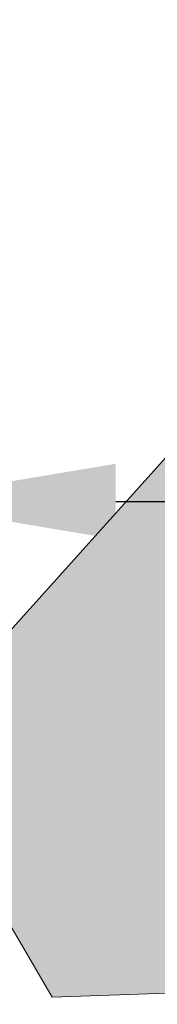
# Model space of a CAD drawing. Units: inches. Extents: x 2091 to 2899, y 967 to 2217.
# Tile 250 of 256: x 2214.58 to 2217.01, y 1131.25 to 1148.63. Entities that reach past the tile are written whole.
import ezdxf

# ---------------------------------------------------------------- set-up
doc = ezdxf.new("R2010")
doc.units = ezdxf.units.IN
doc.layers.add('A-ANNO-DIMS', color=2, linetype='Continuous', lineweight=18)
doc.layers.add('L-PLNT-TREE', color=94, linetype='Continuous', lineweight=13)
doc.layers.add('A-WALL-PATT', color=141, linetype='Continuous', lineweight=13, true_color=0xadddf7)
doc.layers.add('L-PLNT-PATT', color=114, linetype='Continuous', lineweight=13, true_color=0x139b48)
doc.styles.get("Standard").update_dxf_attribs({"font": 'arial.ttf'})
doc.dimstyles.new('ISO-25', dxfattribs={"dimtxt": 4, "dimasz": 4, "dimexe": 1.25, "dimexo": 0.625, "dimtad": 1, "dimdec": 0, "dimlunit": 3, "dimtxsty": 'Standard', "dimcen": 2.5, "dimadec": 0, "dimazin": 0, "dimtfac": 1, "dimtdec": 0, "dimtmove": 0, "dimatfit": 3, "dimfxl": 1, "dimarcsym": 0})

# ---------------------------------------------------------------- blocks, each defined once
blk = doc.blocks.new('*U25')
blk.add_lwpolyline([(-1139.42368, 1783.79628), (-1216.11644, 1685.47796), (-1117.5111, 1601.2033), (-1051.7759, 1643.3419), (-1126.09884, 1521.20092), (-1072.10606, 1527.49758), (-1079.90386, 1416.93646), (-1259.93906, 1179.83508), (-1479.05978, 1165.78888), (-1577.66258, 1109.60662), (-1742.00312, 927.01364), (-1676.26538, 814.64658), (-1270.89408, 828.69278), (-1194.20386, 772.51052), (-1007.95074, 856.78518), (-876.4778, 575.87134), (-821.70016, 575.87134), (-569.71184, 884.87504)])
blk = doc.blocks.new('*D37')
at = {"layer": 'A-ANNO-DIMS', "color": 0, "lineweight": -2, "transparency": 16777216}
for p, q in [((2203.116, 1151.622), (2203.116, 1138.874)), ((2212.276, 1151.622), (2212.276, 1138.874)), ((2199.116, 1140.124), (2195.116, 1140.124)), ((2203.116, 1140.124), (2212.276, 1140.124)), ((2216.276, 1140.124), (2245.908, 1140.124))]:
    blk.add_line(p, q, dxfattribs=at)
at = {"layer": 'A-ANNO-DIMS', "color": 0, "transparency": 16777216}
for points in [[(2199.116, 1140.79), (2199.116, 1139.457), (2203.116, 1140.124)], [(2216.276, 1140.79), (2216.276, 1139.457), (2212.276, 1140.124)]]:
    blk.add_solid(points, dxfattribs=at)
at = {"layer": 'Defpoints', "color": 0, "transparency": 16777216}
for p in [(2203.116, 1152.247), (2212.276, 1152.247), (2212.276, 1140.124)]:
    blk.add_point(p, dxfattribs=at)
at = {"layer": 'A-ANNO-DIMS', "color": 0, "transparency": 16777216, "insert": (2233.092, 1142.791), "char_height": 4, "attachment_point": 5}
blk.add_mtext('0\'-9" TYP.', dxfattribs=at)
blk = doc.blocks.new('*D71')
at = {"layer": 'A-ANNO-DIMS', "color": 0, "lineweight": -2, "transparency": 16777216}
for p, q in [((2212.144, 1351.294), (2212.144, 969.464)), ((2452.144, 1351.294), (2452.144, 969.464)), ((2216.144, 970.714), (2448.144, 970.714))]:
    blk.add_line(p, q, dxfattribs=at)
at = {"layer": 'A-ANNO-DIMS', "color": 0, "transparency": 16777216}
for points in [[(2216.144, 971.381), (2216.144, 970.048), (2212.144, 970.714)], [(2448.144, 971.381), (2448.144, 970.048), (2452.144, 970.714)]]:
    blk.add_solid(points, dxfattribs=at)
at = {"layer": 'Defpoints', "color": 0, "transparency": 16777216}
for p in [(2212.144, 1351.919), (2452.144, 1351.919), (2452.144, 970.714)]:
    blk.add_point(p, dxfattribs=at)
at = {"layer": 'A-ANNO-DIMS', "color": 0, "transparency": 16777216, "insert": (2332.144, 973.382), "char_height": 4, "attachment_point": 5}
blk.add_mtext('20\'-0"', dxfattribs=at)
blk = doc.blocks.new('*D75')
at = {"layer": 'A-ANNO-DIMS', "color": 0, "lineweight": -2, "transparency": 16777216}
for p, q in [((2212.144, 1274.794), (2212.144, 969.464)), ((2308.144, 1274.794), (2308.144, 969.464)), ((2216.144, 970.714), (2304.144, 970.714))]:
    blk.add_line(p, q, dxfattribs=at)
at = {"layer": 'A-ANNO-DIMS', "color": 0, "transparency": 16777216}
for points in [[(2216.144, 971.381), (2216.144, 970.048), (2212.144, 970.714)], [(2304.144, 971.381), (2304.144, 970.048), (2308.144, 970.714)]]:
    blk.add_solid(points, dxfattribs=at)
at = {"layer": 'Defpoints', "color": 0, "transparency": 16777216}
for p in [(2212.144, 1275.419), (2308.144, 1275.419), (2308.144, 970.714)]:
    blk.add_point(p, dxfattribs=at)
at = {"layer": 'A-ANNO-DIMS', "color": 0, "transparency": 16777216, "insert": (2260.144, 973.382), "char_height": 4, "attachment_point": 5}
blk.add_mtext('8\'-0"', dxfattribs=at)

msp = doc.modelspace()

# ---------------------------------------------------------------- hatches: boundary and pattern name
at = {"layer": 'A-WALL-PATT'}
h = msp.add_hatch(color=256, dxfattribs=at)
h.dxf.hatch_style = 1
h.paths.add_polyline_path([(2803.144, 2050.919), (2203.144, 2050.919), (2203.144, 1090.919), (2803.144, 1090.919)])
h.paths.add_polyline_path([(2635.799, 1147.54), (2674.524, 1147.54, 0.376086), (2678.53, 1152.88), (2678.53, 1159.556, 0.333335), (2674.524, 1163.562), (2674.524, 1163.562), (2674.524, 1192.934), (2635.806, 1192.934), (2597.088, 1192.934), (2597.088, 1163.562, 0.333335), (2593.082, 1159.556), (2593.082, 1152.88, 0.376086), (2597.088, 1147.54)], flags=0)
h.paths.add_polyline_path([(2436.01, 1278.241, 0.000483), (2435.953, 1278.215, -0.001328), (2435.936, 1278.112, -0.001711), (2436.116, 1278.041, 0.002185)], flags=0)
h.paths.add_polyline_path([(2794.144, 1143.419), (2794.144, 1347.419), (2543.37, 1347.419), (2543.37, 1351.919), (2794.144, 1351.919), (2794.144, 1392.714), (2793.947, 1392.714), (2793.947, 1473.537), (2794.144, 1473.537), (2794.144, 1531.919), (2650.144, 1531.919), (2650.144, 1536.419), (2794.144, 1536.419), (2794.144, 1692.419), (2609.376, 1692.419), (2609.376, 1644.419), (2604.876, 1644.419), (2604.876, 1744.919), (2609.376, 1744.919), (2609.376, 1696.919), (2794.144, 1696.919), (2794.144, 1780.919), (2609.644, 1780.919), (2493.876, 1780.919), (2493.876, 1785.419), (2609.644, 1785.419), (2794.144, 1785.419), (2794.144, 1847.939), (2793.951, 1847.939), (2793.951, 1928.762), (2794.144, 1928.762), (2794.144, 1941.419), (2614.144, 1941.419), (2614.144, 1821.419), (2609.644, 1821.419), (2609.644, 1941.419), (2392.144, 1941.419), (2392.144, 1819.919), (2387.644, 1819.919), (2387.644, 1941.419), (2212.144, 1941.419), (2212.144, 1783.919), (2392.144, 1783.919), (2392.144, 1780.919), (2212.144, 1780.919), (2212.144, 1629.419), (2387.644, 1629.419), (2387.644, 1744.919), (2392.144, 1744.919), (2392.144, 1627.919), (2317.144, 1627.919), (2317.144, 1551.419), (2317.144, 1536.419), (2459.384, 1536.419), (2459.384, 1602.396), (2463.884, 1602.396), (2463.884, 1531.919), (2456.644, 1531.919), (2456.644, 1529.919), (2452.144, 1529.919), (2452.144, 1531.919), (2312.644, 1531.919), (2312.644, 1551.419), (2306.144, 1551.419), (2306.144, 1555.919), (2308.144, 1555.919), (2308.144, 1551.419), (2312.644, 1551.419), (2312.644, 1627.919), (2212.144, 1627.919), (2212.144, 1555.919), (2270.144, 1555.919), (2270.144, 1551.419), (2212.144, 1551.419), (2212.144, 1351.919), (2272.144, 1351.919), (2272.144, 1347.419), (2212.144, 1347.419), (2212.144, 1275.419), (2308.144, 1275.419), (2308.144, 1351.919), (2452.144, 1351.919), (2452.144, 1493.919), (2456.644, 1493.919), (2456.644, 1347.419), (2312.644, 1347.419), (2312.644, 1270.919), (2212.144, 1270.919), (2212.144, 1099.919), (2281.238, 1099.919), (2282.871, 1110.914), (2282.008, 1116.997), (2278.558, 1121.42), (2268.206, 1128.056), (2272.088, 1128.056), (2273.813, 1131.927), (2279.42, 1134.692), (2285.028, 1135.245), (2287.616, 1137.457), (2288.047, 1138.01), (2289.341, 1140.775), (2291.067, 1139.669), (2292.361, 1135.245), (2295.38, 1136.904), (2296.243, 1135.798), (2297.105, 1133.033), (2300.125, 1138.01), (2303.144, 1138.01), (2304.438, 1135.798), (2303.144, 1133.586), (2306.595, 1134.692), (2307.889, 1133.033), (2310.908, 1135.245), (2313.927, 1134.139), (2315.627, 1132.427), (2308.32, 1117.55), (2290.204, 1109.808), (2288.91, 1103.172), (2289.272, 1099.919), (2434.918, 1099.919), (2431.593, 1124.788), (2429.93, 1169.553), (2430.927, 1240.52), (2435.659, 1238.186), (2437.135, 1196.554), (2438.798, 1143.973), (2442.678, 1111.998), (2446.558, 1099.919), (2794.144, 1099.919), (2794.144, 1138.919), (2548.032, 1138.919), (2548.032, 1143.419), (2548.032, 1148.819), (2546.668, 1148.032), (2528.686, 1179.179, 0.256256), (2512.032, 1148.819), (2512.032, 1143.419), (2512.032, 1138.919), (2507.532, 1138.919), (2507.532, 1143.419), (2507.532, 1148.819, 0.256256), (2490.879, 1179.179), (2472.896, 1148.032), (2471.532, 1148.819), (2471.532, 1143.419), (2467.032, 1143.419), (2467.032, 1269.946, 0.039061), (2460.91, 1273.58), (2467.032, 1273.58), (2467.032, 1286.325, 0.014511), (2465.216, 1286.762), (2467.032, 1287.053), (2467.032, 1323.419), (2471.532, 1323.419), (2471.532, 1148.819), (2489.532, 1179.996), (2490.896, 1179.208), (2490.879, 1179.179, -0.256256), (2507.532, 1148.819), (2507.532, 1143.419), (2512.032, 1143.419), (2512.032, 1148.819, -0.256256), (2528.686, 1179.179), (2528.668, 1179.208), (2530.032, 1179.996), (2548.032, 1148.819), (2548.032, 1143.419)], flags=16)
h.paths.add_polyline_path([(2607.769, 1200.945), (2607.769, 1265.031), (2597.088, 1281.052), (2619.785, 1281.052), (2627.795, 1337.127), (2635.799, 1337.127), (2643.817, 1337.127), (2651.827, 1281.052), (2674.524, 1281.052), (2663.843, 1265.031), (2663.843, 1200.945), (2635.806, 1200.945)], flags=0)
edge = h.paths.add_edge_path(flags=0)
edge.add_ellipse((13303.896, 1272.999), major_axis=(-10595.313, 0), ratio=0.84230387, start_angle=0.6282372, end_angle=0.6465541, ccw=False)
edge.add_ellipse((2711.7, 1156.853), major_axis=(2.22, 0), ratio=0.842304, start_angle=111.5352, end_angle=180.6282, ccw=False)
edge.add_ellipse((13303.156, 1272.999), major_axis=(-10593.026, 0), ratio=0.84230387, start_angle=0.5282715, end_angle=0.6465541, ccw=False)
edge.add_line((2710.765, 1175.333), (2710.13, 1175.333))
edge.add_ellipse((2710.13, 1176.58), major_axis=(1.48, 0), ratio=0.842304, start_angle=180, end_angle=270, ccw=False)
edge.add_line((2708.65, 1176.58), (2708.65, 1200.783))
edge.add_ellipse((2710.13, 1200.783), major_axis=(1.48, 0), ratio=0.842304, start_angle=90, end_angle=180, ccw=False)
edge.add_line((2710.13, 1202.029), (2710.465, 1202.029))
edge.add_ellipse((13303.156, 1272.999), major_axis=(-10593.026, 0), ratio=0.84230387, start_angle=-0.0902291, end_angle=0.3838668, ccw=False)
edge.add_ellipse((2710.13, 1290.927), major_axis=(-1.48, 0), ratio=0.842304, start_angle=0, end_angle=90, ccw=False)
edge.add_line((2708.65, 1290.927), (2708.65, 1315.13))
edge.add_ellipse((2710.13, 1315.13), major_axis=(-1.48, 0), ratio=0.842304, start_angle=-90, end_angle=0, ccw=False)
edge.add_line((2710.13, 1316.377), (2710.706, 1316.377))
edge.add_ellipse((3238.402, 1296.29), major_axis=(528.234, 0), ratio=0.8423039, start_angle=176.34957, end_angle=177.82005, ccw=False)
edge.add_ellipse((2775.063, 1071.451), major_axis=(313.308, 0), ratio=0.8423039, start_angle=102.12597, end_angle=103.78053, ccw=False)
edge.add_ellipse((2775.063, 1078.306), major_axis=(-305.303, 0), ratio=0.8423039, start_angle=-79.79046, end_angle=-77.55537, ccw=False)
edge.add_ellipse((2695.142, 1541.975), major_axis=(-250.96, 0), ratio=0.8423039, start_angle=99.25657, end_angle=102.55493)
edge.add_line((2741.41, 1334.214), (2747.133, 1337.378))
edge.add_ellipse((2747.539, 1336.857), major_axis=(-0.74, 0), ratio=0.842304, start_angle=270, end_angle=307.9331, ccw=False)
edge.add_ellipse((2747.539, 1336.857), major_axis=(-0.74, 0), ratio=0.842304, start_angle=232.0669, end_angle=270, ccw=False)
edge.add_line((2747.945, 1337.378), (2753.667, 1334.214))
edge.add_ellipse((2799.935, 1541.975), major_axis=(250.96, 0), ratio=0.8423039, start_angle=257.44507, end_angle=260.74343)
edge.add_ellipse((2720.014, 1078.306), major_axis=(305.303, 0), ratio=0.8423039, start_angle=77.55537, end_angle=79.79046, ccw=False)
edge.add_ellipse((2720.014, 1071.451), major_axis=(-313.308, 0), ratio=0.8423039, start_angle=256.21947, end_angle=257.87403, ccw=False)
edge.add_ellipse((2256.676, 1296.29), major_axis=(-528.234, 0), ratio=0.8423039, start_angle=182.17995, end_angle=183.65043, ccw=False)
edge.add_line((2784.371, 1316.377), (2784.947, 1316.377))
edge.add_ellipse((2784.947, 1315.13), major_axis=(1.48, 0), ratio=0.842304, start_angle=0, end_angle=90, ccw=False)
edge.add_line((2786.427, 1315.13), (2786.427, 1290.927))
edge.add_ellipse((2784.947, 1290.927), major_axis=(1.48, 0), ratio=0.842304, start_angle=270, end_angle=360, ccw=False)
edge.add_ellipse((-7808.079, 1272.999), major_axis=(10593.026, 0), ratio=0.84230387, start_angle=-0.3838668, end_angle=0.0902291, ccw=False)
edge.add_line((2784.612, 1202.029), (2784.947, 1202.029))
edge.add_ellipse((2784.947, 1200.783), major_axis=(1.48, 0), ratio=0.842304, start_angle=0, end_angle=90, ccw=False)
edge.add_line((2786.427, 1200.783), (2786.427, 1176.58))
edge.add_ellipse((2784.947, 1176.58), major_axis=(-1.48, 0), ratio=0.842304, start_angle=90, end_angle=180, ccw=False)
edge.add_line((2784.947, 1175.333), (2784.313, 1175.333))
edge.add_ellipse((-7808.079, 1272.999), major_axis=(10593.026, 0), ratio=0.84230387, start_angle=-0.6186432, end_angle=-0.5282715, ccw=False)
edge.add_ellipse((2783.377, 1156.853), major_axis=(-2.22, 0), ratio=0.842304, start_angle=179.3718, end_angle=248.4648, ccw=False)
edge.add_ellipse((-7808.819, 1272.999), major_axis=(-10595.313, 0), ratio=0.842303866, start_angle=179.3534459, end_angle=179.3717628, ccw=False)
edge.add_ellipse((2780.297, 1153.501), major_axis=(-5.246, 0), ratio=0.842304, start_angle=90, end_angle=179.3534, ccw=False)
edge.add_line((2780.297, 1149.082), (2714.78, 1149.082))
edge.add_ellipse((2714.78, 1153.501), major_axis=(5.246, 0), ratio=0.842304, start_angle=180.6466, end_angle=270, ccw=False)
edge = h.paths.add_edge_path(flags=0)
edge.add_line((2718.187, 1151.008), (2718.187, 1170.472))
edge.add_ellipse((2721.147, 1170.472), major_axis=(-2.96, 0), ratio=0.842304, start_angle=-90, end_angle=0, ccw=False)
edge.add_line((2721.147, 1172.965), (2773.93, 1172.965))
edge.add_ellipse((2773.93, 1170.472), major_axis=(-2.96, 0), ratio=0.842304, start_angle=180, end_angle=270, ccw=False)
edge.add_line((2776.89, 1170.472), (2776.89, 1151.008))
edge.add_line((2776.89, 1151.008), (2718.187, 1151.008))
edge = h.paths.add_edge_path(flags=0)
edge.add_line((2718.187, 1180.234), (2718.187, 1199.058))
edge.add_ellipse((2747.539, 1320.399), major_axis=(147.018, 0), ratio=0.8423039, start_angle=256.40187, end_angle=283.59813)
edge.add_line((2776.89, 1199.058), (2776.89, 1180.234))
edge.add_ellipse((2747.539, 1301.575), major_axis=(147.018, 0), ratio=0.8423039, start_angle=256.40187, end_angle=283.59813, ccw=False)
edge = h.paths.add_edge_path(flags=0)
edge.add_ellipse((13303.156, 1272.999), major_axis=(-10591.546, 0), ratio=0.84230387, start_angle=0.0555943, end_angle=0.3777642, ccw=False)
edge.add_line((2711.617, 1262.722), (2715.667, 1249.495))
edge.add_ellipse((6413.892, 1241.692), major_axis=(-3698.236, 0), ratio=0.84230387, start_angle=-0.120897, end_angle=0.364076)
edge.add_line((2715.761, 1218.192), (2711.934, 1203.167))
edge = h.paths.add_edge_path(flags=0)
edge.add_line((2718.187, 1251.075), (2716.002, 1267.45))
edge.add_ellipse((2742.151, 1202.19), major_axis=(81.773, 0), ratio=0.842304, start_angle=94.27742, end_angle=111.83495, ccw=False)
edge.add_line((2737.01, 1270.931), (2758.067, 1270.931))
edge.add_ellipse((2752.926, 1202.19), major_axis=(81.773, 0), ratio=0.842304, start_angle=68.16505, end_angle=85.72258, ccw=False)
edge.add_line((2779.075, 1267.45), (2776.89, 1251.075))
edge.add_ellipse((2750.338, 1187.885), major_axis=(79.58, 0), ratio=0.842304, start_angle=67.20809, end_angle=85.12993)
edge.add_line((2756.035, 1254.744), (2739.043, 1254.744))
edge.add_ellipse((2744.739, 1187.885), major_axis=(79.58, 0), ratio=0.842304, start_angle=94.87007, end_angle=112.79191)
edge = h.paths.add_edge_path(flags=0)
edge.add_line((2783.143, 1203.167), (2779.316, 1218.192))
edge.add_ellipse((-918.815, 1241.692), major_axis=(3698.236, 0), ratio=0.84230387, start_angle=-0.364076, end_angle=0.120897)
edge.add_line((2779.41, 1249.495), (2783.46, 1262.722))
edge.add_ellipse((-7808.079, 1272.999), major_axis=(-10591.546, 0), ratio=0.84230387, start_angle=179.6222358, end_angle=179.9444057, ccw=False)
edge = h.paths.add_edge_path(flags=0)
edge.add_ellipse((2734.201, 1286.69), major_axis=(-0.357, 6.34), ratio=0.603834, start_angle=89.002, end_angle=253.6574, ccw=False)
edge.add_line((2730.369, 1286.542), (2730.369, 1301.352))
edge.add_line((2730.369, 1301.352), (2735.913, 1305.215))
edge.add_ellipse((2736.385, 1304.735), major_axis=(0.74, 0), ratio=0.842304, start_angle=90, end_angle=134.4802, ccw=False)
edge.add_line((2736.385, 1305.358), (2738.033, 1305.358))
edge.add_line((2738.033, 1305.358), (2738.033, 1307.708))
edge.add_ellipse((2794.202, 1307.708), major_axis=(56.169, 0), ratio=0.842304, start_angle=150.5614, end_angle=180, ccw=False)
edge.add_ellipse((2700.876, 1307.708), major_axis=(-56.169, 0), ratio=0.842304, start_angle=180, end_angle=209.4386, ccw=False)
edge.add_line((2757.044, 1307.708), (2757.044, 1305.358))
edge.add_line((2757.044, 1305.358), (2758.692, 1305.358))
edge.add_ellipse((2758.692, 1304.735), major_axis=(-0.74, 0), ratio=0.842304, start_angle=225.5198, end_angle=270, ccw=False)
edge.add_line((2759.164, 1305.215), (2764.708, 1301.352))
edge.add_line((2764.708, 1301.352), (2764.708, 1286.542))
edge.add_ellipse((2760.876, 1286.69), major_axis=(0.357, 6.34), ratio=0.603834, start_angle=106.3426, end_angle=270.998, ccw=False)
edge.add_line((2757.044, 1285.797), (2757.044, 1307.708))
edge.add_ellipse((2700.876, 1307.708), major_axis=(-56.169, 0), ratio=0.842304, start_angle=180, end_angle=209.4386)
edge.add_ellipse((2794.202, 1307.708), major_axis=(56.169, 0), ratio=0.842304, start_angle=150.5614, end_angle=180)
edge.add_line((2738.033, 1307.708), (2738.033, 1285.797))
h.paths.add_polyline_path([(2417.812, 1104.45), (2413.492, 1102.53), (2410.612, 1103.97), (2409.172, 1106.37), (2407.252, 1107.33), (2406.292, 1109.73), (2405.332, 1114.05), (2405.332, 1117.89), (2406.292, 1120.13), (2407.252, 1119.81), (2408.848, 1118.328), (2410.174, 1119.424), (2410.211, 1120.406), (2411.041, 1121.419), (2410.699, 1119.859), (2410.174, 1119.424), (2410.088, 1117.176), (2411.133, 1116.206), (2413.972, 1119.33), (2416.852, 1120.77), (2416.87, 1120.799), (2417.035, 1119.405), (2417.896, 1118.143), (2418.292, 1118.37), (2419.544, 1120.039), (2419.361, 1118.387), (2419.032, 1119.356), (2418.399, 1118.512), (2419.252, 1114.53), (2418.794, 1107.199)], flags=0)
h.paths.add_polyline_path([(2508.87, 1347.419), (2508.37, 1347.419), (2508.37, 1351.919), (2508.87, 1351.919)], flags=0)
h.paths.add_polyline_path([(2473.37, 1347.419), (2472.37, 1347.419), (2467.87, 1347.419), (2467.87, 1455.419), (2472.37, 1455.419), (2472.37, 1352.419), (2473.37, 1352.419)], flags=0)
h.paths.add_polyline_path([(2352.106, 1217.446), (2349.226, 1218.886), (2347.786, 1221.286), (2345.866, 1222.246), (2344.906, 1224.646), (2343.946, 1228.966), (2343.946, 1232.806), (2344.906, 1235.046), (2345.866, 1234.726), (2347.462, 1233.244), (2348.788, 1234.341), (2348.825, 1235.322), (2349.655, 1236.336), (2349.313, 1234.775), (2348.788, 1234.341), (2348.702, 1232.093), (2349.747, 1231.123), (2352.586, 1234.246), (2355.466, 1235.686), (2355.484, 1235.715), (2355.649, 1234.322), (2356.51, 1233.06), (2356.906, 1233.286), (2358.158, 1234.956), (2357.975, 1233.304), (2357.646, 1234.273), (2357.013, 1233.428), (2357.866, 1229.446), (2357.408, 1222.115), (2356.426, 1219.366)], flags=0)
h.paths.add_polyline_path([(2348.297, 1112.224), (2347.014, 1112.31), (2345.53, 1114.127), (2345.732, 1115.858), (2346.812, 1116.982), (2346.812, 1114.646), (2345.867, 1114.214), (2346.88, 1114.3)], flags=0)
h.paths.add_polyline_path([(2347.014, 1110.926), (2346.272, 1110.493), (2346.61, 1111.186)], flags=0)
h.paths.add_polyline_path([(2345.867, 1118.194), (2345.53, 1117.329), (2343.708, 1118.021), (2344.383, 1118.626)], flags=0)
h.paths.add_polyline_path([(2346.677, 1109.282), (2346.07, 1108.071), (2345.867, 1110.061)], flags=0)
h.paths.add_polyline_path([(2345.057, 1119.751), (2343.64, 1119.751), (2343.978, 1121.135)], flags=0)
h.paths.add_polyline_path([(2345.26, 1116.55), (2345.125, 1115.858), (2344.922, 1115.685), (2344.72, 1116.377)], flags=0)
h.paths.add_polyline_path([(2345.665, 1112.31), (2345.462, 1111.532), (2344.045, 1111.964), (2344.652, 1112.57)], flags=0)
h.paths.add_polyline_path([(2345.192, 1113.349), (2344.45, 1113.868), (2344.72, 1114.387)], flags=0)
h.paths.add_polyline_path([(2344.652, 1116.809), (2344.18, 1115.685), (2344.652, 1115.339), (2343.91, 1114.906), (2343.033, 1115.944), (2343.64, 1116.463)], flags=0)
h.paths.add_polyline_path([(2345.867, 1106.686), (2344.99, 1105.562), (2344.517, 1106.6)], flags=0)
h.paths.add_polyline_path([(2344.855, 1110.061), (2344.517, 1109.282), (2344.113, 1109.715)], flags=0)
h.paths.add_polyline_path([(2344.045, 1113.522), (2343.438, 1113.089), (2342.763, 1113.954)], flags=0)
h.paths.add_polyline_path([(2344.315, 1111.012), (2342.965, 1110.32), (2342.965, 1111.099)], flags=0)
h.paths.add_polyline_path([(2345.125, 1104.697), (2344.585, 1103.745), (2344.45, 1104.264)], flags=0)
h.paths.add_polyline_path([(2342.83, 1121.222), (2341.75, 1120.53), (2340.536, 1121.049), (2340.131, 1121.828), (2340.671, 1122.952), (2341.143, 1121.828), (2341.615, 1122.001)], flags=0)
h.paths.add_polyline_path([(2342.965, 1119.751), (2343.033, 1118.453), (2342.088, 1118.021), (2342.02, 1119.491)], flags=0)
h.paths.add_polyline_path([(2342.695, 1116.896), (2341.953, 1116.636), (2342.02, 1117.329)], flags=0)
h.paths.add_polyline_path([(2343.033, 1112.224), (2342.02, 1111.791), (2341.548, 1112.224), (2342.358, 1113.349)], flags=0)
h.paths.add_polyline_path([(2343.775, 1104.437), (2342.628, 1102.88), (2342.695, 1104.61), (2343.438, 1105.129)], flags=0)
h.paths.add_polyline_path([(2342.02, 1115.079), (2340.806, 1115.512), (2340.941, 1116.377)], flags=0)
h.paths.add_polyline_path([(2341.481, 1120.097), (2341.481, 1119.405), (2341.076, 1119.578), (2341.143, 1120.097)], flags=0)
h.paths.add_polyline_path([(2341.818, 1114.473), (2340.941, 1113.089), (2340.806, 1114.56)], flags=0)
h.paths.add_polyline_path([(2341.143, 1118.54), (2340.941, 1116.982), (2339.051, 1117.675), (2339.051, 1118.626)], flags=0)
h.paths.add_polyline_path([(2342.695, 1101.668), (2341.953, 1101.841), (2342.56, 1102.361)], flags=0)
h.paths.add_polyline_path([(2340.333, 1119.665), (2338.444, 1119.578), (2337.904, 1120.357), (2339.658, 1120.616)], flags=0)
h.paths.add_polyline_path([(2340.333, 1115.339), (2340.063, 1113.695), (2339.388, 1115.339)], flags=0)
h.paths.add_polyline_path([(2341.818, 1103.831), (2341.548, 1102.88), (2341.143, 1103.658)], flags=0)
h.paths.add_polyline_path([(2339.051, 1122.866), (2337.296, 1121.828), (2337.094, 1123.125), (2337.769, 1123.818)], flags=0)
h.paths.add_polyline_path([(2339.118, 1121.741), (2338.848, 1121.222), (2338.174, 1121.049), (2338.376, 1121.568)], flags=0)
h.paths.add_polyline_path([(2339.186, 1119.319), (2338.646, 1118.713), (2338.241, 1118.107), (2338.241, 1118.886)], flags=0)
h.paths.add_polyline_path([(2341.143, 1101.928), (2340.603, 1101.236), (2340.063, 1101.841), (2340.603, 1102.361)], flags=0)
h.paths.add_polyline_path([(2337.634, 1117.761), (2336.621, 1118.28), (2337.296, 1118.972)], flags=0)
h.paths.add_polyline_path([(2336.824, 1119.578), (2334.799, 1118.972), (2335.204, 1120.357), (2336.554, 1120.876)], flags=0)
h.paths.add_polyline_path([(2339.118, 1100.457), (2337.364, 1100.543), (2336.756, 1101.236)], flags=0)
h.paths.add_polyline_path([(2336.351, 1122.433), (2336.014, 1121.914), (2334.934, 1122.433), (2334.529, 1123.471), (2335.744, 1122.779)], flags=0)
h.paths.add_polyline_path([(2334.732, 1120.876), (2334.259, 1120.357), (2334.057, 1120.789), (2334.597, 1121.308)], flags=0)
h.paths.add_polyline_path([(2334.462, 1122.174), (2332.572, 1121.308), (2331.357, 1122.174), (2332.1, 1122.866)], flags=0)
h.paths.add_polyline_path([(2334.259, 1118.54), (2333.382, 1118.453), (2333.652, 1119.319)], flags=0)
h.paths.add_polyline_path([(2335.542, 1102.274), (2334.192, 1102.62), (2335.272, 1103.312)], flags=0)
h.paths.add_polyline_path([(2332.707, 1119.665), (2331.695, 1120.443), (2332.505, 1120.789)], flags=0)
h.paths.add_polyline_path([(2334.732, 1101.149), (2333.517, 1101.582), (2333.989, 1101.755)], flags=0)
h.paths.add_polyline_path([(2332.64, 1116.636), (2331.087, 1116.29), (2331.965, 1118.194)], flags=0)
h.paths.add_polyline_path([(2330.75, 1121.568), (2330.277, 1120.27), (2328.523, 1119.319), (2328.995, 1121.049)], flags=0)
h.paths.add_polyline_path([(2330.75, 1118.626), (2330.008, 1117.502), (2329.873, 1118.021)], flags=0)
h.paths.add_polyline_path([(2332.1, 1102.361), (2330.547, 1102.014), (2331.695, 1102.966)], flags=0)
h.paths.add_polyline_path([(2329.535, 1113.608), (2329.063, 1112.31), (2328.59, 1113.349)], flags=0)
h.paths.add_polyline_path([(2328.388, 1117.848), (2327.51, 1116.55), (2327.173, 1117.761)], flags=0)
h.paths.add_polyline_path([(2329.738, 1106.513), (2329.535, 1105.302), (2328.253, 1106.081)], flags=0)
h.paths.add_polyline_path([(2328.658, 1114.387), (2328.05, 1114.127), (2328.32, 1114.906)], flags=0)
h.paths.add_polyline_path([(2328.32, 1112.224), (2327.106, 1112.137), (2326.701, 1112.656)], flags=0)
h.paths.add_polyline_path([(2326.903, 1115.252), (2326.701, 1114.127), (2325.216, 1113.608), (2326.093, 1115.339)], flags=0)
h.paths.add_polyline_path([(2326.633, 1108.33), (2326.093, 1107.379), (2325.891, 1108.503), (2326.498, 1109.109)], flags=0)
h.paths.add_polyline_path([(2615.144, 1531.919), (2609.644, 1531.919), (2609.644, 1620.419), (2614.144, 1620.419), (2614.144, 1536.419), (2615.144, 1536.419)], flags=0)
h.paths.add_polyline_path([(2545.144, 1563.419), (2464.144, 1563.419), (2464.144, 1632.419), (2509.144, 1632.419), (2509.144, 1627.919), (2509.144, 1603.919), (2468.644, 1603.919), (2468.644, 1567.919), (2540.644, 1567.919), (2540.644, 1591.919), (2545.144, 1591.919)], flags=0)
h.paths.add_polyline_path([(2388.969, 1549.986), (2357.434, 1549.986), (2357.434, 1623.361), (2399.363, 1623.361), (2435.689, 1623.361), (2435.593, 1602.559), (2435.593, 1602.396), (2388.969, 1602.396)], flags=0)
h.paths.add_polyline_path([(2388.881, 1555.809), (2374.904, 1555.809), (2374.904, 1600.572), (2374.904, 1615.458), (2406.351, 1615.458), (2406.351, 1618.939), (2412.174, 1615.458), (2406.351, 1611.976), (2406.351, 1615.458), (2388.881, 1615.458)], flags=0)
h.paths.add_polyline_path([(2568.876, 1644.419), (2453.376, 1644.419), (2453.376, 1785.419), (2457.876, 1785.419), (2457.876, 1648.919), (2568.876, 1648.919)], flags=0)
h.paths.add_polyline_path([(2212.144, 1945.919), (2212.144, 2041.919), (2794.144, 2041.919), (2794.144, 1945.919)], flags=16)
h.paths.add_polyline_path([(2271.083, 1964.317), (2776.853, 1964.317), (2776.853, 2037.17), (2271.083, 2037.17)], flags=8)
h.paths.add_polyline_path([(2380.649, 1536.824), (2461.041, 1536.824), (2461.041, 1554.653), (2380.649, 1554.653)], flags=8)
h.paths.add_polyline_path([(2240.756, 1609.725), (2309.186, 1609.725), (2309.186, 1617.698), (2240.756, 1617.698)], flags=8)
h.paths.add_polyline_path([(2212.677, 1313.504), (2282.592, 1313.504), (2282.592, 1322.745), (2212.677, 1322.745)], flags=8)
h.paths.add_polyline_path([(2457.112, 1114.779), (2558.482, 1114.779), (2558.482, 1142.22), (2457.112, 1142.22)], flags=8)
h.paths.add_polyline_path([(2473.442, 1273.01), (2604.641, 1273.01), (2604.641, 1318.347), (2473.442, 1318.347)], flags=8)
h.paths.add_polyline_path([(2638.876, 1626.977), (2684.25, 1627.977), (2684.038, 1637.597), (2638.664, 1636.598)], flags=8)
h.paths.add_polyline_path([(2537.591, 1453.793), (2628.39, 1453.793), (2628.39, 1475.345), (2537.591, 1475.345)], flags=8)
h.paths.add_polyline_path([(2504.138, 1714.632), (2554.647, 1714.632), (2554.647, 1730.238), (2504.138, 1730.238)], flags=8)
h.paths.add_polyline_path([(2487.501, 1575.652), (2535.097, 1575.652), (2535.097, 1598.378), (2487.501, 1598.378)], flags=8)
h.paths.add_polyline_path([(2709.099, 1735.71), (2740.017, 1735.71), (2740.017, 1749.938), (2709.099, 1749.938)], flags=8)
h.paths.add_polyline_path([(2442.438, 1792.172), (2564.729, 1792.172), (2564.729, 1842), (2442.438, 1842)], flags=8)
h.paths.add_polyline_path([(2655.816, 1809.644), (2789.52, 1806.694), (2790.085, 1832.292), (2656.381, 1835.242)], flags=8)
h.paths.add_polyline_path([(2234.843, 1797.72), (2368.593, 1794.769), (2369.161, 1820.504), (2235.411, 1823.455)], flags=8)
h.paths.add_polyline_path([(2245.138, 1644.006), (2398.428, 1640.624), (2398.995, 1666.325), (2245.706, 1669.707)], flags=8)
h.paths.add_polyline_path([(2306.143, 1431.169), (2413.768, 1428.794), (2414.333, 1454.392), (2306.708, 1456.766)], flags=8)
h.paths.add_polyline_path([(2306.835, 1458.233), (2393.38, 1456.323), (2393.933, 1481.354), (2307.387, 1483.264)], flags=8)
at = {"layer": 'L-PLNT-PATT'}
h = msp.add_hatch(color=256, dxfattribs=at)
h.dxf.hatch_style = 1
h.paths.add_polyline_path([(2333.338, 1165.659), (2329.024, 1166.212), (2331.612, 1168.424), (2335.063, 1177.271), (2328.162, 1184.46), (2319.535, 1187.225), (2323.417, 1193.308), (2319.966, 1203.814), (2317.809, 1203.814), (2313.496, 1213.215), (2310.908, 1212.662), (2307.889, 1212.662), (2305.732, 1217.086), (2307.026, 1223.168), (2310.477, 1223.168), (2304.007, 1230.91), (2303.136, 1237.046), (2299.693, 1240.864), (2296.674, 1237.546), (2294.949, 1238.652), (2294.517, 1241.417), (2292.361, 1242.523), (2289.341, 1239.758), (2285.89, 1240.311), (2283.302, 1235.334), (2283.302, 1230.91), (2286.753, 1229.251), (2284.165, 1227.592), (2281.577, 1229.804), (2274.244, 1222.615), (2274.244, 1220.957), (2271.225, 1219.298), (2272.088, 1217.639), (2274.244, 1214.321), (2270.362, 1211.556), (2266.48, 1214.321), (2264.324, 1213.768), (2263.461, 1211.556), (2266.48, 1211.003), (2266.912, 1206.579), (2263.539, 1207.132), (2259.579, 1203.261), (2263.892, 1202.708), (2262.167, 1197.178), (2258.285, 1196.625), (2253.971, 1193.861), (2248.795, 1191.096), (2248.364, 1193.308), (2244.482, 1185.013), (2251.383, 1186.672), (2255.697, 1183.907), (2254.403, 1177.271), (2246.639, 1174.506), (2243.188, 1176.718), (2241.894, 1173.4), (2238.875, 1172.847), (2236.287, 1169.53), (2233.267, 1165.659), (2237.149, 1162.341), (2239.737, 1164), (2236.811, 1159.191), (2238.937, 1159.439), (2238.63, 1155.086), (2231.542, 1145.752), (2222.915, 1145.199), (2219.033, 1142.987), (2212.563, 1135.798), (2215.151, 1131.374), (2231.111, 1131.927), (2234.13, 1129.715), (2241.463, 1133.033), (2246.639, 1121.973), (2248.795, 1121.973), (2258.716, 1134.139), (2261.736, 1135.798), (2263.892, 1133.033), (2263.892, 1129.162), (2267.343, 1128.056), (2272.088, 1128.056), (2273.813, 1131.927), (2279.42, 1134.692), (2285.028, 1135.245), (2287.616, 1137.457), (2288.047, 1138.01), (2289.341, 1140.775), (2291.067, 1139.669), (2292.361, 1135.245), (2295.38, 1136.904), (2296.243, 1135.798), (2297.105, 1133.033), (2300.125, 1138.01), (2303.144, 1138.01), (2304.438, 1135.798), (2303.144, 1133.586), (2306.595, 1134.692), (2307.889, 1133.033), (2310.908, 1135.245), (2313.927, 1134.139), (2319.966, 1128.056), (2322.554, 1126.95), (2324.711, 1124.738), (2342.827, 1126.397), (2346.278, 1123.079), (2348.866, 1124.185), (2341.964, 1133.033), (2341.533, 1136.351), (2343.69, 1139.669), (2339.808, 1150.175), (2337.651, 1150.175)])
h.paths.add_polyline_path([(2339.658, 1120.616), (2337.904, 1120.357), (2338.444, 1119.578), (2340.333, 1119.665)])
h.paths.add_polyline_path([(2341.143, 1118.54), (2339.051, 1118.626), (2339.051, 1117.675), (2340.941, 1116.982)])
h.paths.add_polyline_path([(2336.554, 1120.876), (2335.204, 1120.357), (2334.799, 1118.972), (2336.824, 1119.578)])
h.paths.add_polyline_path([(2337.296, 1118.972), (2336.621, 1118.28), (2337.634, 1117.761)])
h.paths.add_polyline_path([(2338.646, 1118.713), (2339.186, 1119.319), (2338.241, 1118.886), (2338.241, 1118.107)])
h.paths.add_polyline_path([(2339.051, 1122.866), (2337.769, 1123.818), (2337.094, 1123.125), (2337.296, 1121.828)])
h.paths.add_polyline_path([(2341.615, 1122.001), (2341.143, 1121.828), (2340.671, 1122.952), (2340.131, 1121.828), (2340.536, 1121.049), (2341.75, 1120.53), (2342.83, 1121.222)])
h.paths.add_polyline_path([(2342.965, 1119.751), (2342.02, 1119.491), (2342.088, 1118.021), (2343.033, 1118.453)])
h.paths.add_polyline_path([(2345.867, 1118.194), (2344.383, 1118.626), (2343.708, 1118.021), (2345.53, 1117.329)])
h.paths.add_polyline_path([(2344.652, 1116.809), (2343.64, 1116.463), (2343.033, 1115.944), (2343.91, 1114.906), (2344.652, 1115.339), (2344.18, 1115.685)])
h.paths.add_polyline_path([(2346.812, 1116.982), (2345.732, 1115.858), (2345.53, 1114.127), (2347.014, 1112.31), (2348.297, 1112.224), (2346.88, 1114.3), (2345.867, 1114.214), (2346.812, 1114.646)])
h.paths.add_polyline_path([(2345.26, 1116.55), (2344.72, 1116.377), (2344.922, 1115.685), (2345.125, 1115.858)])
h.paths.add_polyline_path([(2342.695, 1116.896), (2342.02, 1117.329), (2341.953, 1116.636)])
h.paths.add_polyline_path([(2341.481, 1120.097), (2341.143, 1120.097), (2341.076, 1119.578), (2341.481, 1119.405)])
h.paths.add_polyline_path([(2343.978, 1121.135), (2343.64, 1119.751), (2345.057, 1119.751)])
h.paths.add_polyline_path([(2339.118, 1121.741), (2338.376, 1121.568), (2338.174, 1121.049), (2338.848, 1121.222)])
h.paths.add_polyline_path([(2336.351, 1122.433), (2335.744, 1122.779), (2334.529, 1123.471), (2334.934, 1122.433), (2336.014, 1121.914)])
h.paths.add_polyline_path([(2334.462, 1122.174), (2332.1, 1122.866), (2331.357, 1122.174), (2332.572, 1121.308)])
h.paths.add_polyline_path([(2334.597, 1121.308), (2334.057, 1120.789), (2334.259, 1120.357), (2334.732, 1120.876)])
h.paths.add_polyline_path([(2332.505, 1120.789), (2331.695, 1120.443), (2332.707, 1119.665)])
h.paths.add_polyline_path([(2333.652, 1119.319), (2333.382, 1118.453), (2334.259, 1118.54)])
h.paths.add_polyline_path([(2331.965, 1118.194), (2331.087, 1116.29), (2332.64, 1116.636)])
h.paths.add_polyline_path([(2330.75, 1121.568), (2328.995, 1121.049), (2328.523, 1119.319), (2330.277, 1120.27)])
h.paths.add_polyline_path([(2330.75, 1118.626), (2329.873, 1118.021), (2330.008, 1117.502)])
h.paths.add_polyline_path([(2328.388, 1117.848), (2327.173, 1117.761), (2327.51, 1116.55)])
h.paths.add_polyline_path([(2326.903, 1115.252), (2326.093, 1115.339), (2325.216, 1113.608), (2326.701, 1114.127)])
h.paths.add_polyline_path([(2328.658, 1114.387), (2328.32, 1114.906), (2328.05, 1114.127)])
h.paths.add_polyline_path([(2326.701, 1112.656), (2327.106, 1112.137), (2328.32, 1112.224)])
h.paths.add_polyline_path([(2329.535, 1113.608), (2328.59, 1113.349), (2329.063, 1112.31)])
h.paths.add_polyline_path([(2340.333, 1115.339), (2339.388, 1115.339), (2340.063, 1113.695)])
h.paths.add_polyline_path([(2340.941, 1116.377), (2340.806, 1115.512), (2342.02, 1115.079)])
h.paths.add_polyline_path([(2341.818, 1114.473), (2340.806, 1114.56), (2340.941, 1113.089)])
h.paths.add_polyline_path([(2343.033, 1112.224), (2342.358, 1113.349), (2341.548, 1112.224), (2342.02, 1111.791)])
h.paths.add_polyline_path([(2342.763, 1113.954), (2343.438, 1113.089), (2344.045, 1113.522)])
h.paths.add_polyline_path([(2344.72, 1114.387), (2344.45, 1113.868), (2345.192, 1113.349)])
h.paths.add_polyline_path([(2345.665, 1112.31), (2344.652, 1112.57), (2344.045, 1111.964), (2345.462, 1111.532)])
h.paths.add_polyline_path([(2344.315, 1111.012), (2342.965, 1111.099), (2342.965, 1110.32)])
h.paths.add_polyline_path([(2344.855, 1110.061), (2344.113, 1109.715), (2344.517, 1109.282)])
h.paths.add_polyline_path([(2346.677, 1109.282), (2345.867, 1110.061), (2346.07, 1108.071)])
h.paths.add_polyline_path([(2347.014, 1110.926), (2346.61, 1111.186), (2346.272, 1110.493)])
h.paths.add_polyline_path([(2345.867, 1106.686), (2344.517, 1106.6), (2344.99, 1105.562)])
h.paths.add_polyline_path([(2345.125, 1104.697), (2344.45, 1104.264), (2344.585, 1103.745)])
h.paths.add_polyline_path([(2343.775, 1104.437), (2343.438, 1105.129), (2342.695, 1104.61), (2342.628, 1102.88)])
h.paths.add_polyline_path([(2341.818, 1103.831), (2341.143, 1103.658), (2341.548, 1102.88)])
h.paths.add_polyline_path([(2342.56, 1102.361), (2341.953, 1101.841), (2342.695, 1101.668)])
h.paths.add_polyline_path([(2341.143, 1101.928), (2340.603, 1102.361), (2340.063, 1101.841), (2340.603, 1101.236)])
h.paths.add_polyline_path([(2336.756, 1101.236), (2337.364, 1100.543), (2339.118, 1100.457)])
h.paths.add_polyline_path([(2335.272, 1103.312), (2334.192, 1102.62), (2335.542, 1102.274)])
h.paths.add_polyline_path([(2333.989, 1101.755), (2333.517, 1101.582), (2334.732, 1101.149)])
h.paths.add_polyline_path([(2331.695, 1102.966), (2330.547, 1102.014), (2332.1, 1102.361)])
h.paths.add_polyline_path([(2329.738, 1106.513), (2328.253, 1106.081), (2329.535, 1105.302)])
h.paths.add_polyline_path([(2326.633, 1108.33), (2326.498, 1109.109), (2325.891, 1108.503), (2326.093, 1107.379)])
h.paths.add_polyline_path([(2240.596, 1257.814), (2239.584, 1257.468), (2238.977, 1256.949), (2239.854, 1255.911), (2240.596, 1256.344), (2240.124, 1256.69)])
h.paths.add_polyline_path([(2241.811, 1259.199), (2240.327, 1259.631), (2239.652, 1259.026), (2241.474, 1258.334)])
h.paths.add_polyline_path([(2242.756, 1257.987), (2241.676, 1256.863), (2241.474, 1255.132), (2242.958, 1253.315), (2244.241, 1253.229), (2242.824, 1255.305), (2241.811, 1255.219), (2242.756, 1255.651)])
h.paths.add_polyline_path([(2241.609, 1253.315), (2240.596, 1253.575), (2239.989, 1252.969), (2241.406, 1252.537)])
h.paths.add_polyline_path([(2240.664, 1255.392), (2240.394, 1254.873), (2241.136, 1254.354)])
h.paths.add_polyline_path([(2242.958, 1251.931), (2242.554, 1252.191), (2242.216, 1251.498)])
h.paths.add_polyline_path([(2240.259, 1252.017), (2238.909, 1252.104), (2238.909, 1251.325)])
h.paths.add_polyline_path([(2238.302, 1254.354), (2237.492, 1253.229), (2237.964, 1252.796), (2238.977, 1253.229)])
h.paths.add_polyline_path([(2239.989, 1254.527), (2238.707, 1254.959), (2239.382, 1254.094)])
h.paths.add_polyline_path([(2240.799, 1251.066), (2240.057, 1250.72), (2240.461, 1250.287)])
h.paths.add_polyline_path([(2241.811, 1251.066), (2242.014, 1249.076), (2242.621, 1250.287)])
h.paths.add_polyline_path([(2241.204, 1257.555), (2240.664, 1257.382), (2240.866, 1256.69), (2241.069, 1256.863)])
h.paths.add_polyline_path([(2238.639, 1257.901), (2237.964, 1258.334), (2237.897, 1257.641)])
h.paths.add_polyline_path([(2238.909, 1260.756), (2237.964, 1260.496), (2238.032, 1259.026), (2238.977, 1259.458)])
h.paths.add_polyline_path([(2239.922, 1262.14), (2239.584, 1260.756), (2241.001, 1260.756)])
h.paths.add_polyline_path([(2238.774, 1262.227), (2237.559, 1263.006), (2237.087, 1262.833), (2236.615, 1263.957), (2236.075, 1262.833), (2236.48, 1262.054), (2237.694, 1261.535)])
h.paths.add_polyline_path([(2237.425, 1261.102), (2237.087, 1261.102), (2237.02, 1260.583), (2237.425, 1260.41)])
h.paths.add_polyline_path([(2237.087, 1259.545), (2234.995, 1259.631), (2234.995, 1258.68), (2236.885, 1257.987)])
h.paths.add_polyline_path([(2236.885, 1257.382), (2236.75, 1256.517), (2237.964, 1256.084)])
h.paths.add_polyline_path([(2237.762, 1255.478), (2236.75, 1255.565), (2236.885, 1254.094)])
h.paths.add_polyline_path([(2236.277, 1256.344), (2235.332, 1256.344), (2236.007, 1254.7)])
h.paths.add_polyline_path([(2241.811, 1247.691), (2240.461, 1247.605), (2240.934, 1246.567)])
h.paths.add_polyline_path([(2239.719, 1245.442), (2239.382, 1246.134), (2238.639, 1245.615), (2238.572, 1243.885)])
h.paths.add_polyline_path([(2241.069, 1245.702), (2240.394, 1245.269), (2240.529, 1244.75)])
h.paths.add_polyline_path([(2237.762, 1244.836), (2237.087, 1244.663), (2237.492, 1243.885)])
h.paths.add_polyline_path([(2237.087, 1242.933), (2236.547, 1243.366), (2236.007, 1242.846), (2236.547, 1242.241)])
h.paths.add_polyline_path([(2238.504, 1243.366), (2237.897, 1242.846), (2238.639, 1242.673)])
h.paths.add_polyline_path([(2232.7, 1242.241), (2233.308, 1241.548), (2235.062, 1241.462)], flags=17)
h.paths.add_polyline_path([(2231.216, 1244.317), (2230.136, 1243.625), (2231.486, 1243.279)])
h.paths.add_polyline_path([(2229.933, 1242.76), (2229.461, 1242.587), (2230.676, 1242.154)])
h.paths.add_polyline_path([(2227.639, 1243.971), (2226.491, 1243.019), (2228.044, 1243.366)])
h.paths.add_polyline_path([(2222.577, 1249.335), (2222.442, 1250.114), (2221.835, 1249.508), (2222.037, 1248.384)])
h.paths.add_polyline_path([(2225.682, 1247.518), (2224.197, 1247.086), (2225.479, 1246.307)])
h.paths.add_polyline_path([(2225.479, 1254.613), (2224.534, 1254.354), (2225.007, 1253.315)])
h.paths.add_polyline_path([(2224.264, 1253.229), (2222.645, 1253.661), (2223.05, 1253.142)])
h.paths.add_polyline_path([(2222.847, 1256.257), (2222.037, 1256.344), (2221.16, 1254.613), (2222.645, 1255.132)])
h.paths.add_polyline_path([(2224.332, 1258.853), (2223.117, 1258.766), (2223.454, 1257.555)])
h.paths.add_polyline_path([(2226.694, 1259.631), (2225.817, 1259.026), (2225.952, 1258.507)])
h.paths.add_polyline_path([(2227.909, 1259.199), (2227.031, 1257.295), (2228.584, 1257.641)])
h.paths.add_polyline_path([(2224.264, 1255.911), (2223.994, 1255.132), (2224.602, 1255.392)])
h.paths.add_polyline_path([(2229.596, 1260.324), (2229.326, 1259.458), (2230.203, 1259.545)])
h.paths.add_polyline_path([(2228.449, 1261.794), (2227.639, 1261.448), (2228.651, 1260.67)])
h.paths.add_polyline_path([(2230.406, 1263.179), (2228.044, 1263.871), (2227.301, 1263.179), (2228.516, 1262.313)])
h.paths.add_polyline_path([(2232.768, 1260.583), (2232.498, 1261.881), (2231.148, 1261.362), (2230.743, 1259.977)])
h.paths.add_polyline_path([(2230.676, 1261.881), (2230.541, 1262.313), (2230.001, 1261.794), (2230.203, 1261.362)])
h.paths.add_polyline_path([(2232.295, 1263.438), (2231.688, 1263.784), (2230.473, 1264.476), (2230.878, 1263.438), (2231.958, 1262.919)])
h.paths.add_polyline_path([(2234.995, 1263.871), (2233.713, 1264.823), (2233.038, 1264.13), (2233.24, 1262.833)])
h.paths.add_polyline_path([(2235.062, 1262.746), (2234.32, 1262.573), (2234.118, 1262.054), (2234.792, 1262.227)])
h.paths.add_polyline_path([(2235.602, 1261.621), (2233.848, 1261.362), (2234.388, 1260.583), (2236.277, 1260.67)])
h.paths.add_polyline_path([(2235.13, 1260.324), (2234.185, 1259.891), (2234.185, 1259.112), (2234.59, 1259.718)])
h.paths.add_polyline_path([(2226.694, 1262.573), (2224.939, 1262.054), (2224.467, 1260.324), (2226.221, 1261.275)])
h.paths.add_polyline_path([(2233.24, 1259.977), (2232.565, 1259.285), (2233.578, 1258.766)])
h.paths.add_polyline_path([(2337.267, 1337.827), (2336.187, 1336.703), (2335.985, 1334.972), (2337.469, 1333.155), (2338.752, 1333.069), (2337.335, 1335.145), (2336.322, 1335.059), (2337.267, 1335.491)])
h.paths.add_polyline_path([(2336.322, 1339.039), (2334.838, 1339.471), (2334.163, 1338.866), (2335.985, 1338.174)])
h.paths.add_polyline_path([(2334.433, 1341.98), (2334.095, 1340.596), (2335.512, 1340.596)])
h.paths.add_polyline_path([(2333.285, 1342.067), (2332.07, 1342.846), (2331.598, 1342.673), (2331.126, 1343.797), (2330.586, 1342.673), (2330.991, 1341.894), (2332.205, 1341.375)])
h.paths.add_polyline_path([(2333.42, 1340.596), (2332.475, 1340.336), (2332.543, 1338.866), (2333.488, 1339.298)])
h.paths.add_polyline_path([(2331.936, 1340.942), (2331.598, 1340.942), (2331.531, 1340.423), (2331.936, 1340.25)])
h.paths.add_polyline_path([(2329.573, 1342.586), (2328.831, 1342.413), (2328.629, 1341.894), (2329.303, 1342.067)])
h.paths.add_polyline_path([(2329.506, 1343.711), (2328.224, 1344.663), (2327.549, 1343.97), (2327.751, 1342.673)])
h.paths.add_polyline_path([(2330.113, 1341.461), (2328.359, 1341.202), (2328.899, 1340.423), (2330.788, 1340.51)])
h.paths.add_polyline_path([(2331.598, 1339.385), (2329.506, 1339.471), (2329.506, 1338.52), (2331.396, 1337.827)])
h.paths.add_polyline_path([(2327.009, 1341.721), (2325.659, 1341.202), (2325.254, 1339.817), (2327.279, 1340.423)])
h.paths.add_polyline_path([(2326.806, 1343.278), (2326.199, 1343.624), (2324.984, 1344.316), (2325.389, 1343.278), (2326.469, 1342.759)])
h.paths.add_polyline_path([(2324.917, 1343.019), (2322.555, 1343.711), (2321.812, 1343.019), (2323.027, 1342.153)])
h.paths.add_polyline_path([(2321.205, 1342.413), (2319.45, 1341.894), (2318.978, 1340.164), (2320.732, 1341.115)])
h.paths.add_polyline_path([(2318.843, 1338.693), (2317.628, 1338.606), (2317.965, 1337.395)])
h.paths.add_polyline_path([(2322.42, 1339.039), (2321.542, 1337.135), (2323.095, 1337.481)])
h.paths.add_polyline_path([(2324.107, 1340.164), (2323.837, 1339.298), (2324.714, 1339.385)])
h.paths.add_polyline_path([(2322.96, 1341.634), (2322.15, 1341.288), (2323.162, 1340.51)])
h.paths.add_polyline_path([(2325.187, 1341.721), (2325.052, 1342.153), (2324.512, 1341.634), (2324.714, 1341.202)])
h.paths.add_polyline_path([(2321.205, 1339.471), (2320.328, 1338.866), (2320.463, 1338.347)])
h.paths.add_polyline_path([(2317.358, 1336.097), (2316.548, 1336.184), (2315.671, 1334.453), (2317.156, 1334.972)])
h.paths.add_polyline_path([(2318.775, 1335.751), (2318.505, 1334.972), (2319.113, 1335.232)])
h.paths.add_polyline_path([(2319.99, 1334.453), (2319.045, 1334.194), (2319.518, 1333.155)])
h.paths.add_polyline_path([(2317.156, 1333.501), (2317.561, 1332.982), (2318.775, 1333.069)])
h.paths.add_polyline_path([(2317.088, 1329.175), (2316.953, 1329.954), (2316.346, 1329.348), (2316.548, 1328.224)])
h.paths.add_polyline_path([(2320.193, 1327.358), (2318.708, 1326.926), (2319.99, 1326.147)])
h.paths.add_polyline_path([(2322.15, 1323.811), (2321.002, 1322.859), (2322.555, 1323.206)])
h.paths.add_polyline_path([(2325.727, 1324.157), (2324.647, 1323.465), (2325.997, 1323.119)])
h.paths.add_polyline_path([(2334.23, 1325.282), (2333.893, 1325.974), (2333.15, 1325.455), (2333.083, 1323.725)])
h.paths.add_polyline_path([(2336.322, 1327.531), (2334.972, 1327.445), (2335.445, 1326.407)])
h.paths.add_polyline_path([(2335.31, 1330.906), (2334.568, 1330.56), (2334.972, 1330.127)])
h.paths.add_polyline_path([(2334.77, 1331.857), (2333.42, 1331.944), (2333.42, 1331.165)])
h.paths.add_polyline_path([(2332.813, 1334.194), (2332.003, 1333.069), (2332.475, 1332.636), (2333.488, 1333.069)])
h.paths.add_polyline_path([(2335.107, 1333.415), (2334.5, 1332.809), (2335.917, 1332.377), (2336.12, 1333.155)])
h.paths.add_polyline_path([(2334.635, 1336.53), (2335.107, 1337.654), (2334.095, 1337.308), (2333.488, 1336.789), (2334.365, 1335.751), (2335.107, 1336.184)])
h.paths.add_polyline_path([(2335.715, 1337.395), (2335.175, 1337.222), (2335.377, 1336.53), (2335.58, 1336.703)])
h.paths.add_polyline_path([(2333.15, 1337.741), (2332.475, 1338.174), (2332.408, 1337.481)])
h.paths.add_polyline_path([(2330.788, 1336.184), (2329.843, 1336.184), (2330.518, 1334.54)])
h.paths.add_polyline_path([(2332.273, 1335.318), (2331.261, 1335.405), (2331.396, 1333.934)])
h.paths.add_polyline_path([(2331.396, 1337.222), (2331.261, 1336.357), (2332.475, 1335.924)])
h.paths.add_polyline_path([(2334.5, 1334.367), (2333.218, 1334.799), (2333.893, 1333.934)])
h.paths.add_polyline_path([(2335.175, 1335.232), (2334.905, 1334.713), (2335.647, 1334.194)])
h.paths.add_polyline_path([(2337.132, 1330.127), (2336.322, 1330.906), (2336.525, 1328.916)])
h.paths.add_polyline_path([(2337.065, 1332.031), (2336.727, 1331.338), (2337.469, 1331.771)])
h.paths.add_polyline_path([(2329.641, 1340.164), (2328.696, 1339.731), (2328.696, 1338.952), (2329.101, 1339.558)])
h.paths.add_polyline_path([(2327.751, 1339.817), (2327.076, 1339.125), (2328.089, 1338.606)])
h.paths.add_polyline_path([(2327.211, 1322.081), (2327.819, 1321.388), (2329.573, 1321.302)])
h.paths.add_polyline_path([(2324.444, 1322.6), (2323.972, 1322.427), (2325.187, 1321.994)])
h.paths.add_polyline_path([(2331.058, 1323.206), (2330.518, 1322.686), (2331.058, 1322.081), (2331.598, 1322.773)])
h.paths.add_polyline_path([(2332.273, 1324.676), (2331.598, 1324.503), (2332.003, 1323.725)])
h.paths.add_polyline_path([(2333.015, 1323.206), (2332.408, 1322.686), (2333.15, 1322.513)])
h.paths.add_polyline_path([(2335.58, 1325.542), (2334.905, 1325.109), (2335.04, 1324.59)])
h.paths.add_polyline_path([(2271.083, 1964.317), (2776.853, 1964.317), (2776.853, 2037.17), (2271.083, 2037.17)], flags=9)
h.paths.add_polyline_path([(2380.649, 1536.824), (2461.041, 1536.824), (2461.041, 1554.653), (2380.649, 1554.653)], flags=9)
h.paths.add_polyline_path([(2240.756, 1609.725), (2309.186, 1609.725), (2309.186, 1617.698), (2240.756, 1617.698)], flags=9)
h.paths.add_polyline_path([(2212.677, 1313.504), (2282.592, 1313.504), (2282.592, 1322.745), (2212.677, 1322.745)], flags=9)
h.paths.add_polyline_path([(2457.112, 1114.779), (2558.482, 1114.779), (2558.482, 1142.22), (2457.112, 1142.22)], flags=9)
h.paths.add_polyline_path([(2473.442, 1273.01), (2604.641, 1273.01), (2604.641, 1318.347), (2473.442, 1318.347)], flags=9)
h.paths.add_polyline_path([(2638.876, 1626.977), (2684.25, 1627.977), (2684.038, 1637.597), (2638.664, 1636.598)], flags=9)
h.paths.add_polyline_path([(2537.591, 1453.793), (2628.39, 1453.793), (2628.39, 1475.345), (2537.591, 1475.345)], flags=9)
h.paths.add_polyline_path([(2504.138, 1714.632), (2554.647, 1714.632), (2554.647, 1730.238), (2504.138, 1730.238)], flags=9)
h.paths.add_polyline_path([(2487.501, 1575.652), (2535.097, 1575.652), (2535.097, 1598.378), (2487.501, 1598.378)], flags=9)
h.paths.add_polyline_path([(2709.099, 1735.71), (2740.017, 1735.71), (2740.017, 1749.938), (2709.099, 1749.938)], flags=9)
h.paths.add_polyline_path([(2442.438, 1792.172), (2564.729, 1792.172), (2564.729, 1842), (2442.438, 1842)], flags=9)
h.paths.add_polyline_path([(2655.816, 1809.644), (2789.52, 1806.694), (2790.085, 1832.292), (2656.381, 1835.242)], flags=9)
h.paths.add_polyline_path([(2234.843, 1797.72), (2368.593, 1794.769), (2369.161, 1820.504), (2235.411, 1823.455)], flags=9)
h.paths.add_polyline_path([(2245.138, 1644.006), (2398.428, 1640.624), (2398.995, 1666.325), (2245.706, 1669.707)], flags=9)
h.paths.add_polyline_path([(2306.143, 1431.169), (2413.768, 1428.794), (2414.333, 1454.392), (2306.708, 1456.766)], flags=9)
h.paths.add_polyline_path([(2306.835, 1458.233), (2393.38, 1456.323), (2393.933, 1481.354), (2307.387, 1483.264)], flags=9)

# ---------------------------------------------------------------- block references
at = {"layer": 'L-PLNT-TREE', "xscale": 0.0393700787401575, "yscale": 0.0393700787401575, "zscale": 0.0393700787401575}
msp.add_blockref('*U25', (2281.146, 1099.301), dxfattribs=at)

# ---------------------------------------------------------------- dimensions: what is measured, and where the dimension line sits
at = {"layer": 'A-ANNO-DIMS'}
for base, p1, p2, picture, middle in [((2452.144, 970.714), (2212.144, 1351.919), (2452.144, 1351.919), '*D71', (2332.144, 973.382)), ((2308.144, 970.714), (2212.144, 1275.419), (2308.144, 1275.419), '*D75', (2260.144, 973.382))]:
    dim = msp.add_linear_dim(base=base, p1=p1, p2=p2, dimstyle='ISO-25', override={"dimdec": 1, "dimlfac": 1, "dimrnd": 0, "dimzin": 1, "dimdsep": 46, "dimlunit": 4, "dimfrac": 2}, dxfattribs=at)
    dim.commit()
    dim.dimension.update_dxf_attribs({"geometry": picture, "text_midpoint": middle})
dim = msp.add_linear_dim(base=(2212.276, 1140.124), p1=(2203.116, 1152.247), p2=(2212.276, 1152.247), text='<> TYP.', dimstyle='ISO-25', override={"dimdec": 1, "dimlfac": 1, "dimrnd": 0, "dimzin": 1, "dimdsep": 46, "dimlunit": 4, "dimfrac": 2}, dxfattribs=at)
dim.commit()
dim.dimension.update_dxf_attribs({"geometry": '*D37', "text_midpoint": (2233.092, 1142.791)})

doc.saveas('drawing.dxf')
